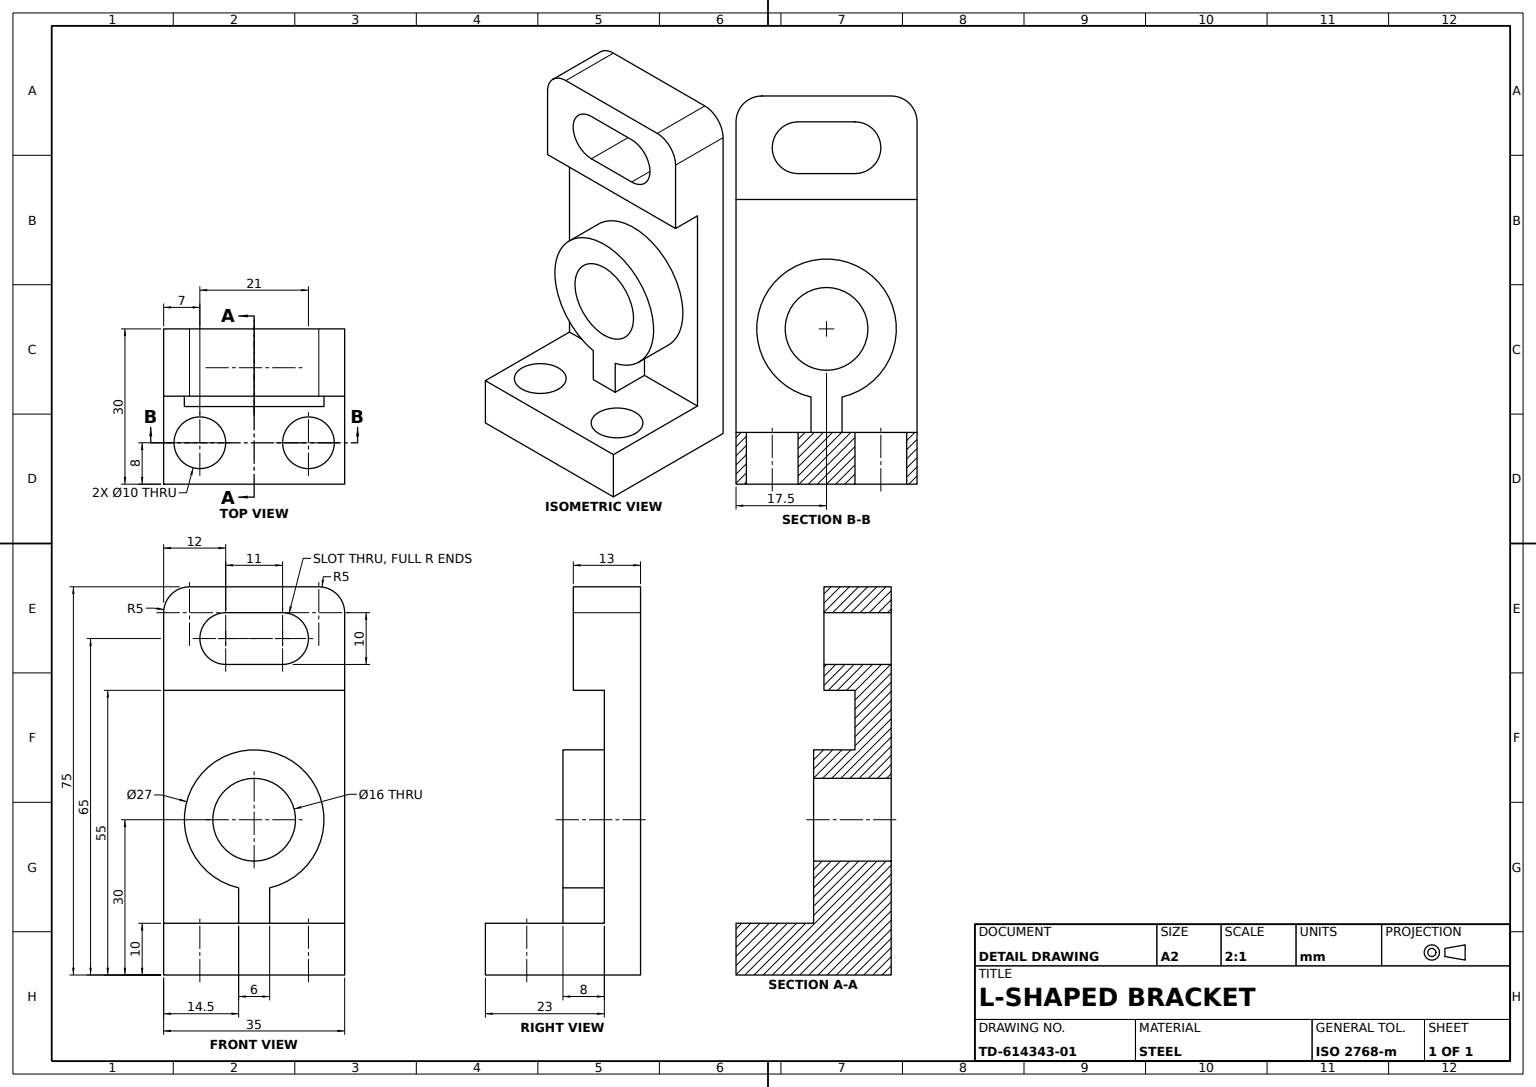
from build123d import *

# Parameters (mm, degrees)
L_BRACKET_BODY_DEPTH     = 17.5
UPRIGHT_TOP_FILLETS_R5_R = 5
BASE_HOLES_REACH         = 75.697
BASE_HOLES_SKETCH_R      = 5
PIVOT_BOSS_SKETCH_R      = 8
PIVOT_BOSS_DEPTH         = 8
PIVOT_BORE_REACH         = 82.376
SKETCH5_2_R              = 8
TOP_SLOT_REACH           = 80.869


with BuildPart() as part:
    # L Bracket Profile Sketch → L Bracket Body (new, symmetric)
    with BuildSketch(Plane.XY):
        Polygon((0, 0), (0, 75), (13, 75), (13, 55), (7, 55), (7, 10), (30, 10), (30, 0), align=None)
    extrude(amount=L_BRACKET_BODY_DEPTH, both=True)

    # Upright Top Fillets R5
    upright_top_fillets_r5_edges = [part.edges().sort_by_distance(p)[0] for p in [
        (6.5, 75, 17.5),
        (6.5, 75, -17.5),
    ]]
    fillet(upright_top_fillets_r5_edges, radius=UPRIGHT_TOP_FILLETS_R5_R)

    # Base Holes Sketch → Base Holes (cut, up to next)
    with BuildSketch(Plane(origin=(0, 10, 0), x_dir=(1, 0, 0), z_dir=(0, 1, 0)), mode=Mode.PRIVATE) as base_holes_sk1:
        with Locations(Location((22, -10.5, 0), (0, 0, 270))):
            Circle(BASE_HOLES_SKETCH_R)
    base_holes_tool1 = extrude(base_holes_sk1.sketch, amount=-BASE_HOLES_REACH, mode=Mode.PRIVATE) & part.part
    # Base Holes Sketch → Base Holes (cut, up to next)
    with BuildSketch(Plane(origin=(0, 10, 0), x_dir=(1, 0, 0), z_dir=(0, 1, 0)), mode=Mode.PRIVATE) as base_holes_sk2:
        with Locations(Location((22, 10.5, 0), (0, 0, 270))):
            Circle(BASE_HOLES_SKETCH_R)
    base_holes_tool2 = extrude(base_holes_sk2.sketch, amount=-BASE_HOLES_REACH, mode=Mode.PRIVATE) & part.part
    add(base_holes_tool1.solids().sort_by_distance((22, 10, 10.5))[0], mode=Mode.SUBTRACT)
    add(base_holes_tool2.solids().sort_by_distance((22, 10, -10.5))[0], mode=Mode.SUBTRACT)

    # Pivot Boss Sketch → Pivot Boss (add)
    with BuildSketch(Plane(origin=(7, 0, 0), x_dir=(0, 0, -1), z_dir=(1, 0, 0))):
        with BuildLine():
            Line((3, 16.837553419), (3, 10))
            Line((3, 10), (-3, 10))
            Line((-3, 10), (-3, 16.837553419))
            ThreePointArc((-3, 16.837553419), (0, 43.5), (3, 16.837553419))
        make_face()
        with Locations(Location((0, 30, 0), (0, 0, 90))):
            Circle(PIVOT_BOSS_SKETCH_R, mode=Mode.SUBTRACT)
    extrude(amount=PIVOT_BOSS_DEPTH)

    # Sketch5_2 → Pivot Bore (cut, up to next)
    with BuildSketch(Plane(origin=(7, 0, 0), x_dir=(0, 0, -1), z_dir=(1, 0, 0)), mode=Mode.PRIVATE) as pivot_bore_sk1:
        with Locations(Location((0, 30, 0), (0, 0, 90))):
            Circle(SKETCH5_2_R)
    pivot_bore_tool1 = extrude(pivot_bore_sk1.sketch, amount=-PIVOT_BORE_REACH, mode=Mode.PRIVATE) & part.part
    add(pivot_bore_tool1.solids().sort_by_distance((7, 30, 0))[0], mode=Mode.SUBTRACT)

    # Top Slot Sketch → Top Slot (cut, up to next)
    with BuildSketch(Plane(origin=(13, 0, 0), x_dir=(0, 0, -1), z_dir=(1, 0, 0)), mode=Mode.PRIVATE) as top_slot_sk1:
        with BuildLine():
            Line((-5.5, 70), (5.5, 70))
            ThreePointArc((5.5, 70), (10.5, 65), (5.5, 60))
            Line((5.5, 60), (-5.5, 60))
            ThreePointArc((-5.5, 60), (-10.5, 65), (-5.5, 70))
        make_face()
    top_slot_tool1 = extrude(top_slot_sk1.sketch, amount=-TOP_SLOT_REACH, mode=Mode.PRIVATE) & part.part
    add(top_slot_tool1.solids().sort_by_distance((13, 65, 0))[0], mode=Mode.SUBTRACT)


solid = part.part
